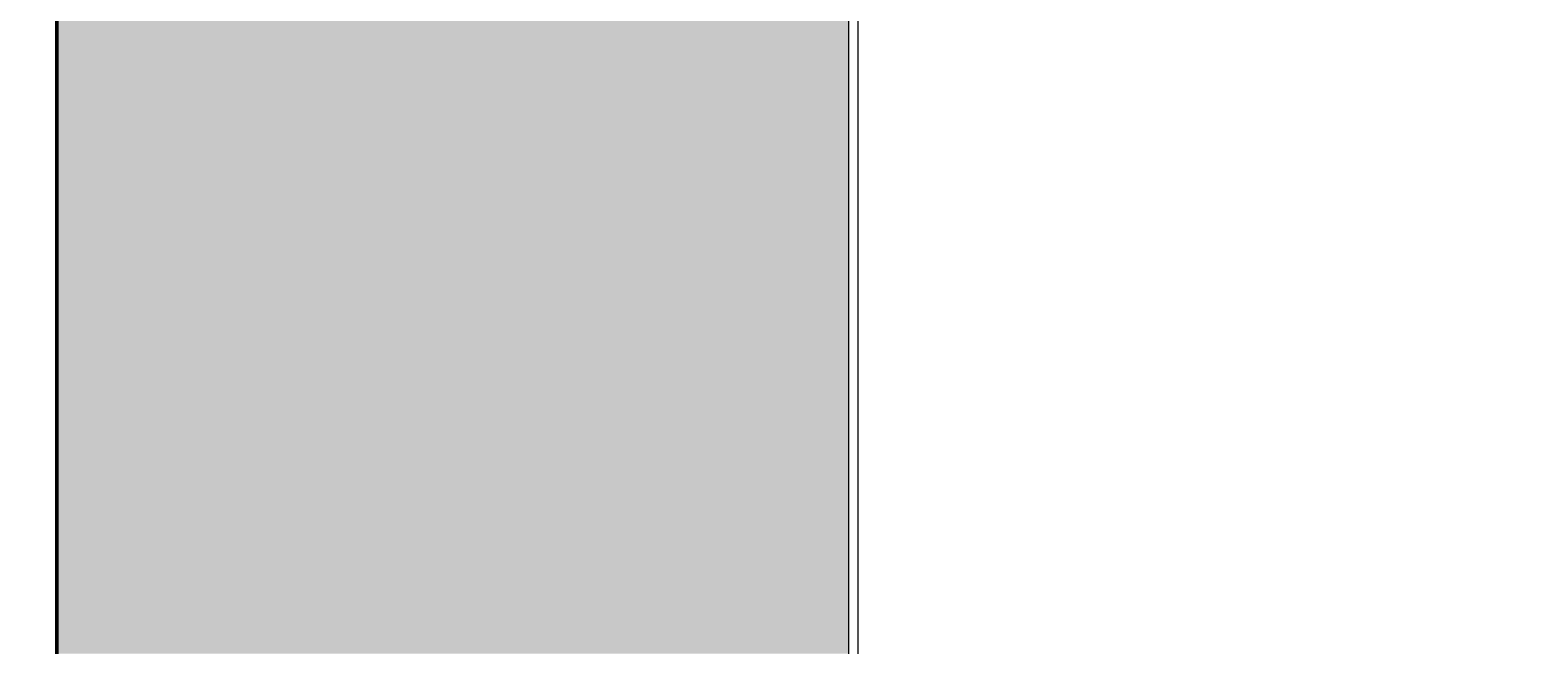
# Model space of a CAD drawing. Units: millimetres. Extents: x 27017497 to 27018854, y 7058029 to 7059154.
# Tile 72 of 91: x 27018319 to 27018360, y 7058207 to 7058224. Entities that reach past the tile are written whole.
import ezdxf

# ---------------------------------------------------------------- set-up
doc = ezdxf.new("R2010")
doc.units = ezdxf.units.MM
for name, color, linetype, lineweight in [('A-ANNO-DIMS', 2, 'Continuous', 18), ('A-FLOR-CASE', 8, 'Continuous', 20), ('A-FLOR-CASE-PATT', 44, 'Continuous', 13), ('A-WALL', 7, 'Continuous', 35)]:
    doc.layers.add(name, color=color, linetype=linetype, lineweight=lineweight)
doc.styles.get("Standard").update_dxf_attribs({"font": 'arial.ttf'})
doc.dimstyles.get("Standard").update_dxf_attribs({"dimtxt": 0.18, "dimasz": 0.18, "dimexe": 0.18, "dimexo": 0.0625, "dimgap": 0.09, "dimtad": 0, "dimtih": 1, "dimtoh": 1, "dimdec": 4, "dimzin": 0, "dimdsep": 46, "dimtxsty": 'Standard', "dimcen": 0.09, "dimadec": 0, "dimazin": 0, "dimtfac": 1, "dimtdec": 4, "dimtofl": 0, "dimtmove": 0, "dimatfit": 3, "dimfxl": 1, "dimtolj": 1, "dimtzin": 0, "dimarcsym": 0})

# ---------------------------------------------------------------- blocks, each defined once
blk = doc.blocks.new('*D47')
at = {"layer": 'A-ANNO-DIMS', "color": 0, "lineweight": -2, "transparency": 16777216}
for p, q in [((27017561.166, 7058294.35), (27017561.166, 7058028.6)), ((27018790.606, 7058294.35), (27018790.606, 7058028.6)), ((27017561.346, 7058028.78), (27018175.431, 7058028.78)), ((27018790.426, 7058028.78), (27018176.341, 7058028.78))]:
    blk.add_line(p, q, dxfattribs=at)
at = {"layer": 'A-ANNO-DIMS', "color": 0, "transparency": 16777216}
for points in [[(27017561.346, 7058028.81), (27017561.346, 7058028.75), (27017561.166, 7058028.78)], [(27018790.426, 7058028.81), (27018790.426, 7058028.75), (27018790.606, 7058028.78)]]:
    blk.add_solid(points, dxfattribs=at)
at = {"layer": 'Defpoints', "color": 0, "transparency": 16777216}
for p in [(27017561.166, 7058294.412), (27018790.606, 7058294.412), (27018790.606, 7058028.78)]:
    blk.add_point(p, dxfattribs=at)
at = {"layer": 'A-ANNO-DIMS', "color": 0, "transparency": 16777216, "insert": (27018175.886, 7058028.78), "char_height": 0.18, "attachment_point": 5}
blk.add_mtext('\\A1;1229.4', dxfattribs=at)
blk = doc.blocks.new('*D48')
at = {"layer": 'A-ANNO-DIMS', "color": 0, "lineweight": -2, "transparency": 16777216}
for p, q in [((27018463.498, 7058622.912), (27017497.536, 7058622.912)), ((27017497.716, 7058622.732), (27017497.716, 7058357.753)), ((27017497.716, 7058092.41), (27017497.716, 7058357.389)), ((27018555.129, 7058092.23), (27017497.536, 7058092.23))]:
    blk.add_line(p, q, dxfattribs=at)
at = {"layer": 'A-ANNO-DIMS', "color": 0, "transparency": 16777216}
for points in [[(27017497.686, 7058622.732), (27017497.746, 7058622.732), (27017497.716, 7058622.912)], [(27017497.686, 7058092.41), (27017497.746, 7058092.41), (27017497.716, 7058092.23)]]:
    blk.add_solid(points, dxfattribs=at)
at = {"layer": 'Defpoints', "color": 0, "transparency": 16777216}
for p in [(27018463.561, 7058622.912), (27017497.716, 7058092.23), (27018555.192, 7058092.23)]:
    blk.add_point(p, dxfattribs=at)
at = {"layer": 'A-ANNO-DIMS', "color": 0, "transparency": 16777216, "insert": (27017497.716, 7058357.571), "char_height": 0.18, "attachment_point": 5}
blk.add_mtext('\\A1;530.7', dxfattribs=at)

msp = doc.modelspace()

# ---------------------------------------------------------------- hatches: boundary and pattern name
at = {"layer": 'A-FLOR-CASE-PATT'}
h = msp.add_hatch(color=256, dxfattribs=at)
h.dxf.hatch_style = 1
edge = h.paths.add_edge_path()
edge.add_line((27018341.343, 7058207.055), (27018330.837, 7058207.055))
edge.add_line((27018330.837, 7058207.055), (27018330.837, 7058203.02))
edge.add_line((27018330.837, 7058203.02), (27018338.424, 7058203.02))
edge.add_ellipse((27018338.23, 7058202.551), major_axis=(0.528, 0), ratio=0.888892, start_angle=0, end_angle=90, ccw=False)
edge.add_line((27018338.758, 7058202.551), (27018338.758, 7058202.238))
edge.add_line((27018338.758, 7058202.238), (27018330.837, 7058201.488))
edge.add_line((27018330.837, 7058201.488), (27018330.837, 7058199.747))
edge.add_line((27018330.837, 7058199.747), (27018338.424, 7058199.747))
edge.add_ellipse((27018338.23, 7058199.277), major_axis=(0.528, 0), ratio=0.888892, start_angle=0, end_angle=90, ccw=False)
edge.add_line((27018338.758, 7058199.277), (27018338.758, 7058198.964))
edge.add_line((27018338.758, 7058198.964), (27018330.837, 7058198.215))
edge.add_line((27018330.837, 7058198.215), (27018330.837, 7058193.415))
edge.add_line((27018330.837, 7058193.415), (27018338.284, 7058190.704))
edge.add_ellipse((27018337.942, 7058190.329), major_axis=(0.496, -0.181), ratio=0.888892, start_angle=0, end_angle=90, ccw=False)
edge.add_line((27018338.439, 7058190.148), (27018338.331, 7058189.854))
edge.add_line((27018338.331, 7058189.854), (27018330.837, 7058191.806))
edge.add_line((27018330.837, 7058191.806), (27018330.837, 7058188.22))
edge.add_line((27018330.837, 7058188.22), (27018338.424, 7058188.22))
edge.add_ellipse((27018338.23, 7058187.75), major_axis=(0.528, 0), ratio=0.888892, start_angle=0, end_angle=90, ccw=False)
edge.add_line((27018338.758, 7058187.75), (27018338.758, 7058187.437))
edge.add_line((27018338.758, 7058187.437), (27018330.837, 7058186.688))
edge.add_line((27018330.837, 7058186.688), (27018330.837, 7058181.982))
edge.add_line((27018330.837, 7058181.982), (27018338.424, 7058181.982))
edge.add_ellipse((27018338.23, 7058181.513), major_axis=(0.528, 0), ratio=0.888892, start_angle=0, end_angle=90, ccw=False)
edge.add_line((27018338.758, 7058181.513), (27018338.758, 7058181.199))
edge.add_line((27018338.758, 7058181.199), (27018330.837, 7058180.45))
edge.add_line((27018330.837, 7058180.45), (27018330.837, 7058178.709))
edge.add_line((27018330.837, 7058178.709), (27018338.424, 7058178.709))
edge.add_ellipse((27018338.23, 7058178.239), major_axis=(0.528, 0), ratio=0.888892, start_angle=0, end_angle=90, ccw=False)
edge.add_line((27018338.758, 7058178.239), (27018338.758, 7058177.926))
edge.add_line((27018338.758, 7058177.926), (27018330.837, 7058177.177))
edge.add_line((27018330.837, 7058177.177), (27018330.837, 7058173.878))
edge.add_line((27018330.837, 7058173.878), (27018338.284, 7058171.167))
edge.add_ellipse((27018337.942, 7058170.792), major_axis=(0.496, -0.181), ratio=0.888892, start_angle=0, end_angle=90, ccw=False)
edge.add_line((27018338.439, 7058170.611), (27018338.331, 7058170.317))
edge.add_line((27018338.331, 7058170.317), (27018330.837, 7058172.269))
edge.add_line((27018330.837, 7058172.269), (27018330.837, 7058168.293))
edge.add_line((27018330.837, 7058168.293), (27018338.424, 7058168.293))
edge.add_ellipse((27018338.23, 7058167.824), major_axis=(0.528, 0), ratio=0.888892, start_angle=0, end_angle=90, ccw=False)
edge.add_line((27018338.758, 7058167.824), (27018338.758, 7058167.511))
edge.add_line((27018338.758, 7058167.511), (27018330.837, 7058166.762))
edge.add_line((27018330.837, 7058166.762), (27018330.837, 7058160.389))
edge.add_line((27018330.837, 7058160.389), (27018338.424, 7058160.389))
edge.add_ellipse((27018338.23, 7058159.92), major_axis=(0.528, 0), ratio=0.888892, start_angle=0, end_angle=90, ccw=False)
edge.add_line((27018338.758, 7058159.92), (27018338.758, 7058159.607))
edge.add_line((27018338.758, 7058159.607), (27018330.837, 7058158.858))
edge.add_line((27018330.837, 7058158.858), (27018330.837, 7058157.116))
edge.add_line((27018330.837, 7058157.116), (27018338.424, 7058157.116))
edge.add_ellipse((27018338.23, 7058156.647), major_axis=(0.528, 0), ratio=0.888892, start_angle=0, end_angle=90, ccw=False)
edge.add_line((27018338.758, 7058156.647), (27018338.758, 7058156.334))
edge.add_line((27018338.758, 7058156.334), (27018330.837, 7058155.585))
edge.add_line((27018330.837, 7058155.585), (27018330.837, 7058150.784))
edge.add_line((27018330.837, 7058150.784), (27018338.284, 7058148.073))
edge.add_ellipse((27018337.942, 7058147.698), major_axis=(0.496, -0.181), ratio=0.888892, start_angle=0, end_angle=90, ccw=False)
edge.add_line((27018338.439, 7058147.517), (27018338.331, 7058147.223))
edge.add_line((27018338.331, 7058147.223), (27018330.837, 7058149.175))
edge.add_line((27018330.837, 7058149.175), (27018330.837, 7058145.589))
edge.add_line((27018330.837, 7058145.589), (27018338.424, 7058145.589))
edge.add_ellipse((27018338.23, 7058145.119), major_axis=(0.528, 0), ratio=0.888892, start_angle=0, end_angle=90, ccw=False)
edge.add_line((27018338.758, 7058145.119), (27018338.758, 7058144.806))
edge.add_line((27018338.758, 7058144.806), (27018330.837, 7058144.057))
edge.add_line((27018330.837, 7058144.057), (27018330.837, 7058141.912))
edge.add_line((27018330.837, 7058141.912), (27018341.343, 7058141.912))
edge.add_line((27018341.343, 7058141.912), (27018341.343, 7058207.055))
edge = h.paths.add_edge_path()
edge.add_line((27018330.112, 7058207.055), (27018319.606, 7058207.055))
edge.add_line((27018319.606, 7058207.055), (27018319.606, 7058141.912))
edge.add_line((27018319.606, 7058141.912), (27018330.112, 7058141.912))
edge.add_line((27018330.112, 7058141.912), (27018330.112, 7058144.024))
edge.add_line((27018330.112, 7058144.024), (27018322.543, 7058144.024))
edge.add_ellipse((27018322.736, 7058144.493), major_axis=(0.528, 0), ratio=0.888892, start_angle=180, end_angle=270, ccw=False)
edge.add_line((27018322.208, 7058144.493), (27018322.208, 7058145.291))
edge.add_ellipse((27018322.736, 7058145.119), major_axis=(0.528, 0), ratio=0.888892, start_angle=90, end_angle=180, ccw=False)
edge.add_line((27018322.736, 7058145.589), (27018330.112, 7058145.589))
edge.add_line((27018330.112, 7058145.589), (27018330.112, 7058149.382))
edge.add_line((27018330.112, 7058149.382), (27018322.826, 7058152.034))
edge.add_ellipse((27018323.168, 7058152.409), major_axis=(0.496, -0.181), ratio=0.888892, start_angle=180, end_angle=270, ccw=False)
edge.add_line((27018322.672, 7058152.59), (27018322.945, 7058153.34))
edge.add_ellipse((27018323.382, 7058152.997), major_axis=(0.496, -0.181), ratio=0.888892, start_angle=90, end_angle=180, ccw=False)
edge.add_line((27018323.543, 7058153.439), (27018330.112, 7058151.048))
edge.add_line((27018330.112, 7058151.048), (27018330.112, 7058155.551))
edge.add_line((27018330.112, 7058155.551), (27018322.543, 7058155.551))
edge.add_ellipse((27018322.736, 7058156.021), major_axis=(0.528, 0), ratio=0.888892, start_angle=180, end_angle=270, ccw=False)
edge.add_line((27018322.208, 7058156.021), (27018322.208, 7058156.819))
edge.add_ellipse((27018322.736, 7058156.647), major_axis=(0.528, 0), ratio=0.888892, start_angle=90, end_angle=180, ccw=False)
edge.add_line((27018322.736, 7058157.116), (27018330.112, 7058157.116))
edge.add_line((27018330.112, 7058157.116), (27018330.112, 7058158.824))
edge.add_line((27018330.112, 7058158.824), (27018322.543, 7058158.824))
edge.add_ellipse((27018322.736, 7058159.294), major_axis=(0.528, 0), ratio=0.888892, start_angle=180, end_angle=270, ccw=False)
edge.add_line((27018322.208, 7058159.294), (27018322.208, 7058160.092))
edge.add_ellipse((27018322.736, 7058159.92), major_axis=(0.528, 0), ratio=0.888892, start_angle=90, end_angle=180, ccw=False)
edge.add_line((27018322.736, 7058160.389), (27018330.112, 7058160.389))
edge.add_line((27018330.112, 7058160.389), (27018330.112, 7058166.728))
edge.add_line((27018330.112, 7058166.728), (27018322.543, 7058166.728))
edge.add_ellipse((27018322.736, 7058167.198), major_axis=(0.528, 0), ratio=0.888892, start_angle=180, end_angle=270, ccw=False)
edge.add_line((27018322.208, 7058167.198), (27018322.208, 7058167.996))
edge.add_ellipse((27018322.736, 7058167.824), major_axis=(0.528, 0), ratio=0.888892, start_angle=90, end_angle=180, ccw=False)
edge.add_line((27018322.736, 7058168.293), (27018330.112, 7058168.293))
edge.add_line((27018330.112, 7058168.293), (27018330.112, 7058172.476))
edge.add_line((27018330.112, 7058172.476), (27018322.826, 7058175.128))
edge.add_ellipse((27018323.168, 7058175.503), major_axis=(0.496, -0.181), ratio=0.888892, start_angle=180, end_angle=270, ccw=False)
edge.add_line((27018322.672, 7058175.684), (27018322.945, 7058176.433))
edge.add_ellipse((27018323.382, 7058176.091), major_axis=(0.496, -0.181), ratio=0.888892, start_angle=90, end_angle=180, ccw=False)
edge.add_line((27018323.543, 7058176.533), (27018330.112, 7058174.142))
edge.add_line((27018330.112, 7058174.142), (27018330.112, 7058177.144))
edge.add_line((27018330.112, 7058177.144), (27018322.543, 7058177.144))
edge.add_ellipse((27018322.736, 7058177.613), major_axis=(0.528, 0), ratio=0.888892, start_angle=180, end_angle=270, ccw=False)
edge.add_line((27018322.208, 7058177.613), (27018322.208, 7058178.411))
edge.add_ellipse((27018322.736, 7058178.239), major_axis=(0.528, 0), ratio=0.888892, start_angle=90, end_angle=180, ccw=False)
edge.add_line((27018322.736, 7058178.709), (27018330.112, 7058178.709))
edge.add_line((27018330.112, 7058178.709), (27018330.112, 7058180.417))
edge.add_line((27018330.112, 7058180.417), (27018322.543, 7058180.417))
edge.add_ellipse((27018322.736, 7058180.886), major_axis=(0.528, 0), ratio=0.888892, start_angle=180, end_angle=270, ccw=False)
edge.add_line((27018322.208, 7058180.886), (27018322.208, 7058181.684))
edge.add_ellipse((27018322.736, 7058181.513), major_axis=(0.528, 0), ratio=0.888892, start_angle=90, end_angle=180, ccw=False)
edge.add_line((27018322.736, 7058181.982), (27018330.112, 7058181.982))
edge.add_line((27018330.112, 7058181.982), (27018330.112, 7058186.655))
edge.add_line((27018330.112, 7058186.655), (27018322.543, 7058186.655))
edge.add_ellipse((27018322.736, 7058187.124), major_axis=(0.528, 0), ratio=0.888892, start_angle=180, end_angle=270, ccw=False)
edge.add_line((27018322.208, 7058187.124), (27018322.208, 7058187.922))
edge.add_ellipse((27018322.736, 7058187.75), major_axis=(0.528, 0), ratio=0.888892, start_angle=90, end_angle=180, ccw=False)
edge.add_line((27018322.736, 7058188.22), (27018330.112, 7058188.22))
edge.add_line((27018330.112, 7058188.22), (27018330.112, 7058192.013))
edge.add_line((27018330.112, 7058192.013), (27018322.826, 7058194.665))
edge.add_ellipse((27018323.168, 7058195.04), major_axis=(0.496, -0.181), ratio=0.888892, start_angle=180, end_angle=270, ccw=False)
edge.add_line((27018322.672, 7058195.22), (27018322.945, 7058195.97))
edge.add_ellipse((27018323.382, 7058195.628), major_axis=(0.496, -0.181), ratio=0.888892, start_angle=90, end_angle=180, ccw=False)
edge.add_line((27018323.543, 7058196.069), (27018330.112, 7058193.678))
edge.add_line((27018330.112, 7058193.678), (27018330.112, 7058198.182))
edge.add_line((27018330.112, 7058198.182), (27018322.543, 7058198.182))
edge.add_ellipse((27018322.736, 7058198.651), major_axis=(0.528, 0), ratio=0.888892, start_angle=180, end_angle=270, ccw=False)
edge.add_line((27018322.208, 7058198.651), (27018322.208, 7058199.449))
edge.add_ellipse((27018322.736, 7058199.277), major_axis=(0.528, 0), ratio=0.888892, start_angle=90, end_angle=180, ccw=False)
edge.add_line((27018322.736, 7058199.747), (27018330.112, 7058199.747))
edge.add_line((27018330.112, 7058199.747), (27018330.112, 7058201.455))
edge.add_line((27018330.112, 7058201.455), (27018322.543, 7058201.455))
edge.add_ellipse((27018322.736, 7058201.924), major_axis=(0.528, 0), ratio=0.888892, start_angle=180, end_angle=270, ccw=False)
edge.add_line((27018322.208, 7058201.924), (27018322.208, 7058202.722))
edge.add_ellipse((27018322.736, 7058202.551), major_axis=(0.528, 0), ratio=0.888892, start_angle=90, end_angle=180, ccw=False)
edge.add_line((27018322.736, 7058203.02), (27018330.112, 7058203.02))
edge.add_line((27018330.112, 7058203.02), (27018330.112, 7058207.055))
h.paths.add_polyline_path([(27018341.31, 7058294.412), (27018319.606, 7058294.412), (27018319.606, 7058207.1), (27018341.31, 7058207.1)])
h.paths.add_polyline_path([(27018354.358, 7058255.592), (27018354.358, 7058256.057, -0.414214), (27018354.869, 7058256.569), (27018346.477, 7058256.569, -0.414214), (27018345.197, 7058257.848), (27018345.197, 7058259.128, -0.414214), (27018346.477, 7058260.407), (27018343.868, 7058260.407, 0.290979), (27018341.551, 7058258.934), (27018341.551, 7058242.534, 0.290979), (27018343.868, 7058241.06), (27018346.477, 7058241.06, -0.414214), (27018345.197, 7058242.34), (27018345.197, 7058243.619, -0.414214), (27018346.477, 7058244.899), (27018353.078, 7058244.899, 0.414214), (27018354.358, 7058246.178)])
h.paths.add_polyline_path([(27018356.917, 7058260.407), (27018346.477, 7058260.407, 0.414214), (27018345.197, 7058259.128), (27018345.197, 7058257.848, 0.414214), (27018346.477, 7058256.569), (27018355.637, 7058256.569), (27018355.637, 7058244.899), (27018346.477, 7058244.899, 0.414214), (27018345.197, 7058243.619), (27018345.197, 7058242.34, 0.414214), (27018346.477, 7058241.06), (27018356.917, 7058241.06, 0.414214), (27018359.476, 7058243.619), (27018359.476, 7058257.848, 0.414214)])
h.paths.add_polyline_path([(27018355.637, 7058252.362), (27018355.637, 7058256.057, 0.490314), (27018354.997, 7058256.553, 0.490314), (27018354.358, 7058256.057), (27018354.358, 7058255.592), (27018354.358, 7058245.411, 0.490314), (27018354.997, 7058244.915, 0.490314), (27018355.637, 7058245.411)], flags=17)

# ---------------------------------------------------------------- linework, layer by layer
at = {"layer": 'A-FLOR-CASE'}
for p, q in [((27018341.31, 7058207.055), (27018341.31, 7058294.412)), ((27018341.551, 7058290.392), (27018341.551, 7058203.035)), ((27018319.573, 7058207.055), (27018319.573, 7058251.237))]:
    msp.add_line(p, q, dxfattribs=at)
at = {"layer": 'A-WALL'}
msp.add_line((27018319.606, 7058386.803), (27018319.606, 7058141.912), dxfattribs=at)

# ---------------------------------------------------------------- dimensions: what is measured, and where the dimension line sits
at = {"layer": 'A-ANNO-DIMS'}
dim = msp.add_linear_dim(base=(27017497.716, 7058092.23), p1=(27018463.561, 7058622.912), p2=(27018555.192, 7058092.23), angle=90, dimstyle='Standard', override={"dimdec": 1, "dimlfac": 1, "dimrnd": 0, "dimzin": 0, "dimdsep": 46, "dimlunit": 2}, dxfattribs=at)
dim.commit()
dim.dimension.update_dxf_attribs({"geometry": '*D48', "text_midpoint": (27017497.716, 7058357.571)})
dim = msp.add_linear_dim(base=(27018790.606, 7058028.78), p1=(27017561.166, 7058294.412), p2=(27018790.606, 7058294.412), dimstyle='Standard', override={"dimdec": 1, "dimlfac": 1, "dimrnd": 0, "dimzin": 0, "dimdsep": 46, "dimlunit": 2}, dxfattribs=at)
dim.commit()
dim.dimension.update_dxf_attribs({"geometry": '*D47', "text_midpoint": (27018175.886, 7058028.78)})

doc.saveas('drawing.dxf')
